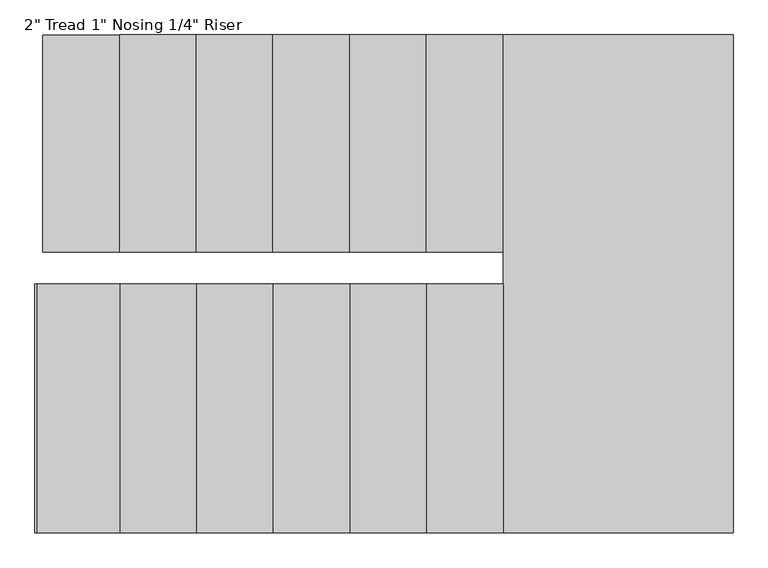
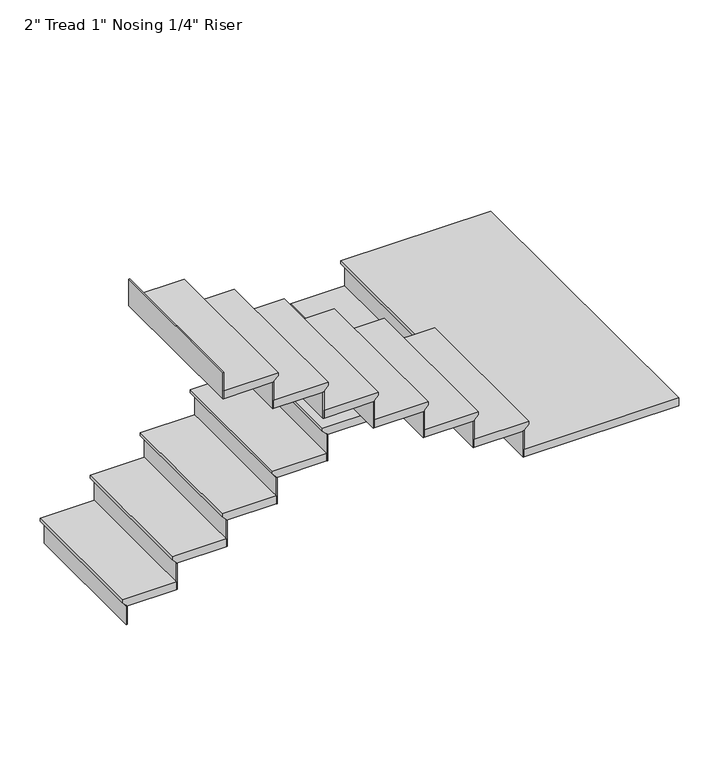
"""IFC4 building model written with IfcOpenShell, lengths in millimetres: stair flight geometry."""

from ifc_helpers import new_model, si_unit, origin, place, context, project, spatial, faceted_brep, source, transform, mapped, element, save


def stair_flight_fe7d2e61(model_context):
    return source(origin(), model_context, "Body", "Brep", [
        faceted_brep([(-879.540747, -2928.9064015, 3350.6833333), (-879.540747, -2928.9064015, 3369.7333333), (-879.540747, -2065.3064015, 3369.7333333), (-879.540747, -2065.3064015, 3350.6833333), (-854.140747, -2928.9064015, 3325.2833333), (-854.140747, -2065.3064015, 3325.2833333), (-549.340747, -2928.9064015, 3369.7333333), (-549.340747, -2065.3064015, 3369.7333333), (-854.140747, -2065.3064015, 3318.9333333), (-549.340747, -2065.3064015, 3318.9333333), (-549.340747, -2928.9064015, 3318.9333333), (-854.140747, -2928.9064015, 3318.9333333)], [[[0, 1, 2, 3]], [[4, 0, 3, 5]], [[2, 1, 6, 7]], [[8, 9, 10, 11]], [[2, 7, 9, 8, 5, 3]], [[8, 11, 4, 5]], [[6, 1, 0, 4, 11, 10]], [[7, 6, 10, 9]]]),
        faceted_brep([(-854.140747, -2928.9064015, 3318.9333333), (-854.140747, -2928.9064015, 3200.4), (-847.790747, -2928.9064015, 3200.4), (-847.790747, -2928.9064015, 3318.9333333), (-854.140747, -2065.3064015, 3318.9333333), (-847.790747, -2065.3064015, 3318.9333333), (-847.790747, -2065.3064015, 3200.4), (-854.140747, -2065.3064015, 3200.4)], [[[0, 1, 2, 3]], [[4, 5, 6, 7]], [[1, 0, 4, 7]], [[2, 1, 7, 6]], [[3, 2, 6, 5]], [[0, 3, 5, 4]]]),
        faceted_brep([(-549.340747, -2928.9064015, 3488.2666667), (-549.340747, -2928.9064015, 3318.9333333), (-542.990747, -2928.9064015, 3318.9333333), (-542.990747, -2928.9064015, 3488.2666667), (-549.340747, -2065.3064015, 3488.2666667), (-542.990747, -2065.3064015, 3488.2666667), (-542.990747, -2065.3064015, 3318.9333333), (-549.340747, -2065.3064015, 3318.9333333)], [[[0, 1, 2, 3]], [[4, 5, 6, 7]], [[1, 0, 4, 7]], [[2, 1, 7, 6]], [[3, 2, 6, 5]], [[0, 3, 5, 4]]]),
        faceted_brep([(-574.740747, -2065.3064015, 3539.0666667), (-574.740747, -2928.9064015, 3539.0666667), (-244.540747, -2928.9064015, 3539.0666667), (-244.540747, -2065.3064015, 3539.0666667), (-549.340747, -2065.3064015, 3488.2666667), (-244.540747, -2065.3064015, 3488.2666667), (-244.540747, -2928.9064015, 3488.2666667), (-549.340747, -2928.9064015, 3488.2666667), (-549.340747, -2065.3064015, 3494.6166667), (-574.740747, -2065.3064015, 3520.0166667), (-549.340747, -2928.9064015, 3494.6166667), (-574.740747, -2928.9064015, 3520.0166667)], [[[0, 1, 2, 3]], [[4, 5, 6, 7]], [[0, 3, 5, 4, 8, 9]], [[4, 7, 10, 8]], [[2, 1, 11, 10, 7, 6]], [[3, 2, 6, 5]], [[11, 1, 0, 9]], [[10, 11, 9, 8]]]),
        faceted_brep([(-244.540747, -2928.9064015, 3657.6), (-244.540747, -2928.9064015, 3488.2666667), (-238.190747, -2928.9064015, 3488.2666667), (-238.190747, -2928.9064015, 3657.6), (-244.540747, -2065.3064015, 3657.6), (-238.190747, -2065.3064015, 3657.6), (-238.190747, -2065.3064015, 3488.2666667), (-244.540747, -2065.3064015, 3488.2666667)], [[[0, 1, 2, 3]], [[4, 5, 6, 7]], [[1, 0, 4, 7]], [[2, 1, 7, 6]], [[3, 2, 6, 5]], [[0, 3, 5, 4]]]),
        faceted_brep([(-269.940747, -2065.3064015, 3708.4), (-269.940747, -2928.9064015, 3708.4), (60.259253, -2928.9064015, 3708.4), (60.259253, -2065.3064015, 3708.4), (-244.540747, -2065.3064015, 3657.6), (60.259253, -2065.3064015, 3657.6), (60.259253, -2928.9064015, 3657.6), (-244.540747, -2928.9064015, 3657.6), (-244.540747, -2065.3064015, 3663.95), (-269.940747, -2065.3064015, 3689.35), (-244.540747, -2928.9064015, 3663.95), (-269.940747, -2928.9064015, 3689.35)], [[[0, 1, 2, 3]], [[4, 5, 6, 7]], [[0, 3, 5, 4, 8, 9]], [[4, 7, 10, 8]], [[2, 1, 11, 10, 7, 6]], [[3, 2, 6, 5]], [[11, 1, 0, 9]], [[10, 11, 9, 8]]]),
        faceted_brep([(60.259253, -2928.9064015, 3826.9333333), (60.259253, -2928.9064015, 3657.6), (66.609253, -2928.9064015, 3657.6), (66.609253, -2928.9064015, 3826.9333333), (60.259253, -2065.3064015, 3826.9333333), (66.609253, -2065.3064015, 3826.9333333), (66.609253, -2065.3064015, 3657.6), (60.259253, -2065.3064015, 3657.6)], [[[0, 1, 2, 3]], [[4, 5, 6, 7]], [[1, 0, 4, 7]], [[2, 1, 7, 6]], [[3, 2, 6, 5]], [[0, 3, 5, 4]]]),
        faceted_brep([(34.859253, -2065.3064015, 3877.7333333), (34.859253, -2928.9064015, 3877.7333333), (365.059253, -2928.9064015, 3877.7333333), (365.059253, -2065.3064015, 3877.7333333), (60.259253, -2065.3064015, 3826.9333333), (365.059253, -2065.3064015, 3826.9333333), (365.059253, -2928.9064015, 3826.9333333), (60.259253, -2928.9064015, 3826.9333333), (60.259253, -2065.3064015, 3833.2833333), (34.859253, -2065.3064015, 3858.6833333), (60.259253, -2928.9064015, 3833.2833333), (34.859253, -2928.9064015, 3858.6833333)], [[[0, 1, 2, 3]], [[4, 5, 6, 7]], [[0, 3, 5, 4, 8, 9]], [[4, 7, 10, 8]], [[2, 1, 11, 10, 7, 6]], [[3, 2, 6, 5]], [[11, 1, 0, 9]], [[10, 11, 9, 8]]]),
        faceted_brep([(365.059253, -2928.9064015, 3996.2666667), (365.059253, -2928.9064015, 3826.9333333), (371.409253, -2928.9064015, 3826.9333333), (371.409253, -2928.9064015, 3996.2666667), (365.059253, -2065.3064015, 3996.2666667), (371.409253, -2065.3064015, 3996.2666667), (371.409253, -2065.3064015, 3826.9333333), (365.059253, -2065.3064015, 3826.9333333)], [[[0, 1, 2, 3]], [[4, 5, 6, 7]], [[1, 0, 4, 7]], [[2, 1, 7, 6]], [[3, 2, 6, 5]], [[0, 3, 5, 4]]]),
        faceted_brep([(339.659253, -2065.3064015, 4047.0666667), (339.659253, -2928.9064015, 4047.0666667), (669.859253, -2928.9064015, 4047.0666667), (669.859253, -2065.3064015, 4047.0666667), (365.059253, -2065.3064015, 3996.2666667), (669.859253, -2065.3064015, 3996.2666667), (669.859253, -2928.9064015, 3996.2666667), (365.059253, -2928.9064015, 3996.2666667), (365.059253, -2065.3064015, 4002.6166667), (339.659253, -2065.3064015, 4028.0166667), (365.059253, -2928.9064015, 4002.6166667), (339.659253, -2928.9064015, 4028.0166667)], [[[0, 1, 2, 3]], [[4, 5, 6, 7]], [[0, 3, 5, 4, 8, 9]], [[4, 7, 10, 8]], [[2, 1, 11, 10, 7, 6]], [[3, 2, 6, 5]], [[11, 1, 0, 9]], [[10, 11, 9, 8]]]),
        faceted_brep([(669.859253, -2928.9064015, 4165.6), (669.859253, -2928.9064015, 3996.2666667), (676.209253, -2928.9064015, 3996.2666667), (676.209253, -2928.9064015, 4165.6), (669.859253, -2065.3064015, 4165.6), (676.209253, -2065.3064015, 4165.6), (676.209253, -2065.3064015, 3996.2666667), (669.859253, -2065.3064015, 3996.2666667)], [[[0, 1, 2, 3]], [[4, 5, 6, 7]], [[1, 0, 4, 7]], [[2, 1, 7, 6]], [[3, 2, 6, 5]], [[0, 3, 5, 4]]]),
        faceted_brep([(644.459253, -2065.3064015, 4216.4), (644.459253, -2928.9064015, 4216.4), (974.659253, -2928.9064015, 4216.4), (974.659253, -2065.3064015, 4216.4), (669.859253, -2065.3064015, 4165.6), (974.659253, -2065.3064015, 4165.6), (974.659253, -2928.9064015, 4165.6), (669.859253, -2928.9064015, 4165.6), (669.859253, -2065.3064015, 4171.95), (644.459253, -2065.3064015, 4197.35), (669.859253, -2928.9064015, 4171.95), (644.459253, -2928.9064015, 4197.35)], [[[0, 1, 2, 3]], [[4, 5, 6, 7]], [[0, 3, 5, 4, 8, 9]], [[4, 7, 10, 8]], [[2, 1, 11, 10, 7, 6]], [[3, 2, 6, 5]], [[11, 1, 0, 9]], [[10, 11, 9, 8]]]),
        faceted_brep([(974.659253, -2928.9064015, 4334.9333333), (974.659253, -2928.9064015, 4165.6), (981.009253, -2928.9064015, 4165.6), (981.009253, -2928.9064015, 4334.9333333), (974.659253, -2065.3064015, 4334.9333333), (981.009253, -2065.3064015, 4334.9333333), (981.009253, -2065.3064015, 4165.6), (974.659253, -2065.3064015, 4165.6)], [[[0, 1, 2, 3]], [[4, 5, 6, 7]], [[1, 0, 4, 7]], [[2, 1, 7, 6]], [[3, 2, 6, 5]], [[0, 3, 5, 4]]]),
        faceted_brep([(923.859253, -4046.5064015, 4385.7333333), (1863.659253, -4046.5064015, 4385.7333333), (1863.659253, -2065.3064015, 4385.7333333), (949.259253, -2065.3064015, 4385.7333333), (949.259253, -3055.9064015, 4385.7333333), (923.859253, -3055.9064015, 4385.7333333), (1863.659253, -4046.5064015, 4334.9333333), (923.859253, -4046.5064015, 4334.9333333), (923.859253, -3055.9064015, 4334.9333333), (949.259253, -3055.9064015, 4334.9333333), (949.259253, -2928.9064015, 4334.9333333), (974.659253, -2928.9064015, 4334.9333333), (974.659253, -2065.3064015, 4334.9333333), (1863.659253, -2065.3064015, 4334.9333333), (974.659253, -2065.3064015, 4341.2833333), (949.259253, -2065.3064015, 4366.6833333), (974.659253, -2928.9064015, 4341.2833333), (949.259253, -2928.9064015, 4366.6833333)], [[[0, 1, 2, 3, 4, 5]], [[6, 7, 8, 9, 10, 11, 12, 13]], [[1, 0, 7, 6]], [[2, 1, 6, 13]], [[3, 2, 13, 12, 14, 15]], [[12, 11, 16, 14]], [[11, 10, 17, 16]], [[4, 3, 15, 17, 10, 9]], [[5, 4, 9, 8]], [[0, 5, 8, 7]], [[15, 14, 16, 17]]]),
        faceted_brep([(923.859253, -3055.9064015, 4504.2666667), (923.859253, -3055.9064015, 4334.9333333), (917.509253, -3055.9064015, 4334.9333333), (917.509253, -3055.9064015, 4504.2666667), (923.859253, -4046.5064015, 4504.2666667), (917.509253, -4046.5064015, 4504.2666667), (917.509253, -4046.5064015, 4334.9333333), (923.859253, -4046.5064015, 4334.9333333)], [[[0, 1, 2, 3]], [[4, 5, 6, 7]], [[1, 0, 4, 7]], [[2, 1, 7, 6]], [[3, 2, 6, 5]], [[0, 3, 5, 4]]]),
        faceted_brep([(949.259253, -4046.5064015, 4555.0666667), (949.259253, -3055.9064015, 4555.0666667), (619.059253, -3055.9064015, 4555.0666667), (619.059253, -4046.5064015, 4555.0666667), (923.859253, -4046.5064015, 4504.2666667), (619.059253, -4046.5064015, 4504.2666667), (619.059253, -3055.9064015, 4504.2666667), (923.859253, -3055.9064015, 4504.2666667), (923.859253, -4046.5064015, 4510.6166667), (949.259253, -4046.5064015, 4536.0166667), (923.859253, -3055.9064015, 4510.6166667), (949.259253, -3055.9064015, 4536.0166667)], [[[0, 1, 2, 3]], [[4, 5, 6, 7]], [[0, 3, 5, 4, 8, 9]], [[4, 7, 10, 8]], [[2, 1, 11, 10, 7, 6]], [[3, 2, 6, 5]], [[11, 1, 0, 9]], [[10, 11, 9, 8]]]),
        faceted_brep([(619.059253, -3055.9064015, 4673.6), (619.059253, -3055.9064015, 4504.2666667), (612.709253, -3055.9064015, 4504.2666667), (612.709253, -3055.9064015, 4673.6), (619.059253, -4046.5064015, 4673.6), (612.709253, -4046.5064015, 4673.6), (612.709253, -4046.5064015, 4504.2666667), (619.059253, -4046.5064015, 4504.2666667)], [[[0, 1, 2, 3]], [[4, 5, 6, 7]], [[1, 0, 4, 7]], [[2, 1, 7, 6]], [[3, 2, 6, 5]], [[0, 3, 5, 4]]]),
        faceted_brep([(644.459253, -4046.5064015, 4724.4), (644.459253, -3055.9064015, 4724.4), (314.259253, -3055.9064015, 4724.4), (314.259253, -4046.5064015, 4724.4), (619.059253, -4046.5064015, 4673.6), (314.259253, -4046.5064015, 4673.6), (314.259253, -3055.9064015, 4673.6), (619.059253, -3055.9064015, 4673.6), (619.059253, -4046.5064015, 4679.95), (644.459253, -4046.5064015, 4705.35), (619.059253, -3055.9064015, 4679.95), (644.459253, -3055.9064015, 4705.35)], [[[0, 1, 2, 3]], [[4, 5, 6, 7]], [[0, 3, 5, 4, 8, 9]], [[4, 7, 10, 8]], [[2, 1, 11, 10, 7, 6]], [[3, 2, 6, 5]], [[11, 1, 0, 9]], [[10, 11, 9, 8]]]),
        faceted_brep([(314.259253, -3055.9064015, 4842.9333333), (314.259253, -3055.9064015, 4673.6), (307.909253, -3055.9064015, 4673.6), (307.909253, -3055.9064015, 4842.9333333), (314.259253, -4046.5064015, 4842.9333333), (307.909253, -4046.5064015, 4842.9333333), (307.909253, -4046.5064015, 4673.6), (314.259253, -4046.5064015, 4673.6)], [[[0, 1, 2, 3]], [[4, 5, 6, 7]], [[1, 0, 4, 7]], [[2, 1, 7, 6]], [[3, 2, 6, 5]], [[0, 3, 5, 4]]]),
        faceted_brep([(339.659253, -4046.5064015, 4893.7333333), (339.659253, -3055.9064015, 4893.7333333), (9.459253, -3055.9064015, 4893.7333333), (9.459253, -4046.5064015, 4893.7333333), (314.259253, -4046.5064015, 4842.9333333), (9.459253, -4046.5064015, 4842.9333333), (9.459253, -3055.9064015, 4842.9333333), (314.259253, -3055.9064015, 4842.9333333), (314.259253, -4046.5064015, 4849.2833333), (339.659253, -4046.5064015, 4874.6833333), (314.259253, -3055.9064015, 4849.2833333), (339.659253, -3055.9064015, 4874.6833333)], [[[0, 1, 2, 3]], [[4, 5, 6, 7]], [[0, 3, 5, 4, 8, 9]], [[4, 7, 10, 8]], [[2, 1, 11, 10, 7, 6]], [[3, 2, 6, 5]], [[11, 1, 0, 9]], [[10, 11, 9, 8]]]),
        faceted_brep([(9.459253, -3055.9064015, 5012.2666667), (9.459253, -3055.9064015, 4842.9333333), (3.109253, -3055.9064015, 4842.9333333), (3.109253, -3055.9064015, 5012.2666667), (9.459253, -4046.5064015, 5012.2666667), (3.109253, -4046.5064015, 5012.2666667), (3.109253, -4046.5064015, 4842.9333333), (9.459253, -4046.5064015, 4842.9333333)], [[[0, 1, 2, 3]], [[4, 5, 6, 7]], [[1, 0, 4, 7]], [[2, 1, 7, 6]], [[3, 2, 6, 5]], [[0, 3, 5, 4]]]),
        faceted_brep([(34.859253, -4046.5064015, 5063.0666667), (34.859253, -3055.9064015, 5063.0666667), (-295.340747, -3055.9064015, 5063.0666667), (-295.340747, -4046.5064015, 5063.0666667), (9.459253, -4046.5064015, 5012.2666667), (-295.340747, -4046.5064015, 5012.2666667), (-295.340747, -3055.9064015, 5012.2666667), (9.459253, -3055.9064015, 5012.2666667), (9.459253, -4046.5064015, 5018.6166667), (34.859253, -4046.5064015, 5044.0166667), (9.459253, -3055.9064015, 5018.6166667), (34.859253, -3055.9064015, 5044.0166667)], [[[0, 1, 2, 3]], [[4, 5, 6, 7]], [[0, 3, 5, 4, 8, 9]], [[4, 7, 10, 8]], [[2, 1, 11, 10, 7, 6]], [[3, 2, 6, 5]], [[11, 1, 0, 9]], [[10, 11, 9, 8]]]),
        faceted_brep([(-295.340747, -3055.9064015, 5181.6), (-295.340747, -3055.9064015, 5012.2666667), (-301.690747, -3055.9064015, 5012.2666667), (-301.690747, -3055.9064015, 5181.6), (-295.340747, -4046.5064015, 5181.6), (-301.690747, -4046.5064015, 5181.6), (-301.690747, -4046.5064015, 5012.2666667), (-295.340747, -4046.5064015, 5012.2666667)], [[[0, 1, 2, 3]], [[4, 5, 6, 7]], [[1, 0, 4, 7]], [[2, 1, 7, 6]], [[3, 2, 6, 5]], [[0, 3, 5, 4]]]),
        faceted_brep([(-269.940747, -4046.5064015, 5232.4), (-269.940747, -3055.9064015, 5232.4), (-600.140747, -3055.9064015, 5232.4), (-600.140747, -4046.5064015, 5232.4), (-295.340747, -4046.5064015, 5181.6), (-600.140747, -4046.5064015, 5181.6), (-600.140747, -3055.9064015, 5181.6), (-295.340747, -3055.9064015, 5181.6), (-295.340747, -4046.5064015, 5187.95), (-269.940747, -4046.5064015, 5213.35), (-295.340747, -3055.9064015, 5187.95), (-269.940747, -3055.9064015, 5213.35)], [[[0, 1, 2, 3]], [[4, 5, 6, 7]], [[0, 3, 5, 4, 8, 9]], [[4, 7, 10, 8]], [[2, 1, 11, 10, 7, 6]], [[3, 2, 6, 5]], [[11, 1, 0, 9]], [[10, 11, 9, 8]]]),
        faceted_brep([(-600.140747, -3055.9064015, 5350.9333333), (-600.140747, -3055.9064015, 5181.6), (-606.490747, -3055.9064015, 5181.6), (-606.490747, -3055.9064015, 5350.9333333), (-600.140747, -4046.5064015, 5350.9333333), (-606.490747, -4046.5064015, 5350.9333333), (-606.490747, -4046.5064015, 5181.6), (-600.140747, -4046.5064015, 5181.6)], [[[0, 1, 2, 3]], [[4, 5, 6, 7]], [[1, 0, 4, 7]], [[2, 1, 7, 6]], [[3, 2, 6, 5]], [[0, 3, 5, 4]]]),
        faceted_brep([(-904.940747, -3055.9064015, 5520.2666667), (-904.940747, -3055.9064015, 5350.9333333), (-911.290747, -3055.9064015, 5350.9333333), (-911.290747, -3055.9064015, 5520.2666667), (-904.940747, -4046.5064015, 5520.2666667), (-911.290747, -4046.5064015, 5520.2666667), (-911.290747, -4046.5064015, 5350.9333333), (-904.940747, -4046.5064015, 5350.9333333)], [[[0, 1, 2, 3]], [[4, 5, 6, 7]], [[1, 0, 4, 7]], [[2, 1, 7, 6]], [[3, 2, 6, 5]], [[0, 3, 5, 4]]]),
        faceted_brep([(-574.740747, -4046.5064015, 5401.7333333), (-574.740747, -3055.9064015, 5401.7333333), (-904.940747, -3055.9064015, 5401.7333333), (-904.940747, -4046.5064015, 5401.7333333), (-600.140747, -4046.5064015, 5350.9333333), (-904.940747, -4046.5064015, 5350.9333333), (-904.940747, -3055.9064015, 5350.9333333), (-600.140747, -3055.9064015, 5350.9333333), (-600.140747, -4046.5064015, 5357.2833333), (-574.740747, -4046.5064015, 5382.6833333), (-600.140747, -3055.9064015, 5357.2833333), (-574.740747, -3055.9064015, 5382.6833333)], [[[0, 1, 2, 3]], [[4, 5, 6, 7]], [[0, 3, 5, 4, 8, 9]], [[4, 7, 10, 8]], [[2, 1, 11, 10, 7, 6]], [[3, 2, 6, 5]], [[11, 1, 0, 9]], [[10, 11, 9, 8]]]),
    ])


if __name__ == "__main__":
    model = new_model("IFC4")
    model_context = context("Model", 3, world=origin())
    ifc_project = project(units=[si_unit("LENGTHUNIT", "METRE", prefix="MILLI")], contexts=[model_context])
    site = spatial("IfcSite", under=ifc_project)
    building = spatial("IfcBuilding", under=site)
    placement = place(None, origin())
    stair_flight_shape = stair_flight_fe7d2e61(model_context)
    element("IfcStairFlight", 1, ObjectType="2\" Tread 1\" Nosing 1/4\" Riser", at=placement, inside=building, context=model_context, shape_type="MappedRepresentation", body=[
        mapped(stair_flight_shape, transform((0.0, 0.0, 0.0), x_axis=(1.0, 0.0, 0.0), y_axis=(0.0, 1.0, 0.0), z_axis=(0.0, 0.0, 1.0))),
    ])
    save(model, "model.ifc")
